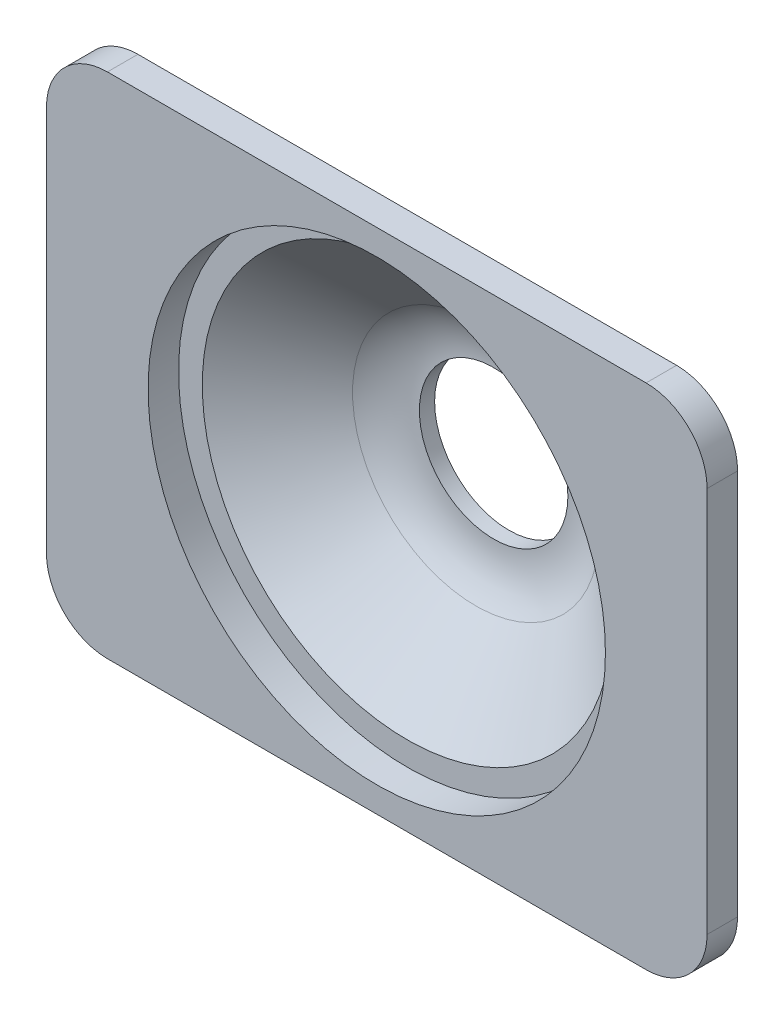
ISO-10303-21;
HEADER;
FILE_DESCRIPTION(('STEP AP214'),'2;1');
FILE_NAME('part.step','',(''),(''),'','','');
FILE_SCHEMA(('AUTOMOTIVE_DESIGN { 1 0 10303 214 1 1 1 1 }'));
ENDSEC;
DATA;
#1=APPLICATION_CONTEXT('core data for automotive mechanical design processes');
#2=APPLICATION_PROTOCOL_DEFINITION('international standard','automotive_design',2000,#1);
#3=PRODUCT_CONTEXT('',#1,'mechanical');
#4=PRODUCT('Part','Part','',(#3));
#5=PRODUCT_RELATED_PRODUCT_CATEGORY('part','',(#4));
#6=PRODUCT_DEFINITION_FORMATION('','',#4);
#7=PRODUCT_DEFINITION_CONTEXT('part definition',#1,'design');
#8=PRODUCT_DEFINITION('design','',#6,#7);
#9=PRODUCT_DEFINITION_SHAPE('','',#8);
#10=(LENGTH_UNIT() NAMED_UNIT(*) SI_UNIT(.MILLI.,.METRE.));
#11=(NAMED_UNIT(*) PLANE_ANGLE_UNIT() SI_UNIT($,.RADIAN.));
#12=(NAMED_UNIT(*) SI_UNIT($,.STERADIAN.) SOLID_ANGLE_UNIT());
#13=UNCERTAINTY_MEASURE_WITH_UNIT(LENGTH_MEASURE(1.E-05),#10,'distance_accuracy_value','');
#14=(GEOMETRIC_REPRESENTATION_CONTEXT(3) GLOBAL_UNCERTAINTY_ASSIGNED_CONTEXT((#13)) GLOBAL_UNIT_ASSIGNED_CONTEXT((#10,
#11,#12)) REPRESENTATION_CONTEXT('',''));
#15=CARTESIAN_POINT('',(0.,0.,0.));
#16=DIRECTION('',(0.,0.,1.));
#17=DIRECTION('',(1.,0.,0.));
#18=AXIS2_PLACEMENT_3D('',#15,#16,#17);
#19=CARTESIAN_POINT('',(-26.5,-19.,3.));
#20=DIRECTION('',(0.,0.,-1.));
#21=DIRECTION('',(-1.,0.,0.));
#22=AXIS2_PLACEMENT_3D('',#19,#20,#21);
#23=PLANE('',#22);
#24=CARTESIAN_POINT('',(-26.5,-19.,3.));
#25=DIRECTION('',(0.,0.,1.));
#26=DIRECTION('',(-1.,0.,0.));
#27=AXIS2_PLACEMENT_3D('',#24,#25,#26);
#28=CIRCLE('',#27,6.);
#29=CARTESIAN_POINT('',(-32.5,-19.,3.));
#30=VERTEX_POINT('',#29);
#31=CARTESIAN_POINT('',(-26.5,-25.,3.));
#32=VERTEX_POINT('',#31);
#33=EDGE_CURVE('E152',#30,#32,#28,.T.);
#34=ORIENTED_EDGE('',*,*,#33,.T.);
#35=DIRECTION('',(1.,0.,0.));
#36=VECTOR('',#35,1.);
#37=CARTESIAN_POINT('',(-26.5,-25.,3.));
#38=LINE('',#37,#36);
#39=CARTESIAN_POINT('',(26.5,-25.,3.));
#40=VERTEX_POINT('',#39);
#41=EDGE_CURVE('E100',#32,#40,#38,.T.);
#42=ORIENTED_EDGE('',*,*,#41,.T.);
#43=CARTESIAN_POINT('',(26.5,-19.,3.));
#44=DIRECTION('',(0.,0.,1.));
#45=DIRECTION('',(1.,0.,0.));
#46=AXIS2_PLACEMENT_3D('',#43,#44,#45);
#47=CIRCLE('',#46,6.);
#48=CARTESIAN_POINT('',(32.5,-19.,3.));
#49=VERTEX_POINT('',#48);
#50=EDGE_CURVE('E168',#40,#49,#47,.T.);
#51=ORIENTED_EDGE('',*,*,#50,.T.);
#52=DIRECTION('',(0.,1.,0.));
#53=VECTOR('',#52,1.);
#54=CARTESIAN_POINT('',(32.5,-19.,3.));
#55=LINE('',#54,#53);
#56=CARTESIAN_POINT('',(32.5,19.,3.));
#57=VERTEX_POINT('',#56);
#58=EDGE_CURVE('E178',#49,#57,#55,.T.);
#59=ORIENTED_EDGE('',*,*,#58,.T.);
#60=CARTESIAN_POINT('',(26.5,19.,3.));
#61=DIRECTION('',(0.,0.,1.));
#62=DIRECTION('',(-1.,0.,0.));
#63=AXIS2_PLACEMENT_3D('',#60,#61,#62);
#64=CIRCLE('',#63,6.);
#65=CARTESIAN_POINT('',(26.5,25.,3.));
#66=VERTEX_POINT('',#65);
#67=EDGE_CURVE('E117',#57,#66,#64,.T.);
#68=ORIENTED_EDGE('',*,*,#67,.T.);
#69=DIRECTION('',(-1.,0.,0.));
#70=VECTOR('',#69,1.);
#71=CARTESIAN_POINT('',(-26.5,25.,3.));
#72=LINE('',#71,#70);
#73=CARTESIAN_POINT('',(-26.5,25.,3.));
#74=VERTEX_POINT('',#73);
#75=EDGE_CURVE('E115',#66,#74,#72,.T.);
#76=ORIENTED_EDGE('',*,*,#75,.T.);
#77=CARTESIAN_POINT('',(-26.5,19.,3.));
#78=DIRECTION('',(0.,0.,1.));
#79=DIRECTION('',(-1.,0.,0.));
#80=AXIS2_PLACEMENT_3D('',#77,#78,#79);
#81=CIRCLE('',#80,6.);
#82=CARTESIAN_POINT('',(-32.5,19.,3.));
#83=VERTEX_POINT('',#82);
#84=EDGE_CURVE('E116',#74,#83,#81,.T.);
#85=ORIENTED_EDGE('',*,*,#84,.T.);
#86=DIRECTION('',(0.,-1.,0.));
#87=VECTOR('',#86,1.);
#88=CARTESIAN_POINT('',(-32.5,-19.,3.));
#89=LINE('',#88,#87);
#90=EDGE_CURVE('E57',#83,#30,#89,.T.);
#91=ORIENTED_EDGE('',*,*,#90,.T.);
#92=EDGE_LOOP('',(#34,#42,#51,#59,#68,#76,#85,#91));
#93=FACE_BOUND('',#92,.T.);
#94=CARTESIAN_POINT('',(0.,0.,3.));
#95=DIRECTION('',(0.,0.,1.));
#96=DIRECTION('',(1.,0.,0.));
#97=AXIS2_PLACEMENT_3D('',#94,#95,#96);
#98=CIRCLE('',#97,22.5);
#99=CARTESIAN_POINT('',(22.5,0.,3.));
#100=VERTEX_POINT('',#99);
#101=EDGE_CURVE('E137',#100,#100,#98,.T.);
#102=ORIENTED_EDGE('',*,*,#101,.F.);
#103=EDGE_LOOP('',(#102));
#104=FACE_BOUND('',#103,.T.);
#105=ADVANCED_FACE('F39',(#93,#104),#23,.F.);
#106=CARTESIAN_POINT('',(-26.5,-19.,0.));
#107=DIRECTION('',(0.,0.,-1.));
#108=DIRECTION('',(-1.,0.,0.));
#109=AXIS2_PLACEMENT_3D('',#106,#107,#108);
#110=PLANE('',#109);
#111=CARTESIAN_POINT('',(0.,0.,0.));
#112=DIRECTION('',(0.,0.,1.));
#113=DIRECTION('',(1.,0.,0.));
#114=AXIS2_PLACEMENT_3D('',#111,#112,#113);
#115=CIRCLE('',#114,24.6838214055972);
#116=CARTESIAN_POINT('',(24.6838214055972,0.,0.));
#117=VERTEX_POINT('',#116);
#118=EDGE_CURVE('E204',#117,#117,#115,.T.);
#119=ORIENTED_EDGE('',*,*,#118,.T.);
#120=EDGE_LOOP('',(#119));
#121=FACE_BOUND('',#120,.T.);
#122=CARTESIAN_POINT('',(-26.5,-19.,0.));
#123=DIRECTION('',(0.,0.,1.));
#124=DIRECTION('',(-1.,0.,0.));
#125=AXIS2_PLACEMENT_3D('',#122,#123,#124);
#126=CIRCLE('',#125,6.);
#127=CARTESIAN_POINT('',(-32.5,-19.,0.));
#128=VERTEX_POINT('',#127);
#129=CARTESIAN_POINT('',(-26.5,-25.,0.));
#130=VERTEX_POINT('',#129);
#131=EDGE_CURVE('E139',#128,#130,#126,.T.);
#132=ORIENTED_EDGE('',*,*,#131,.F.);
#133=DIRECTION('',(0.,-1.,0.));
#134=VECTOR('',#133,1.);
#135=CARTESIAN_POINT('',(-32.5,-19.,0.));
#136=LINE('',#135,#134);
#137=CARTESIAN_POINT('',(-32.5,19.,0.));
#138=VERTEX_POINT('',#137);
#139=EDGE_CURVE('E94',#138,#128,#136,.T.);
#140=ORIENTED_EDGE('',*,*,#139,.F.);
#141=CARTESIAN_POINT('',(-26.5,19.,0.));
#142=DIRECTION('',(0.,0.,1.));
#143=DIRECTION('',(-1.,0.,0.));
#144=AXIS2_PLACEMENT_3D('',#141,#142,#143);
#145=CIRCLE('',#144,6.);
#146=CARTESIAN_POINT('',(-26.5,25.,0.));
#147=VERTEX_POINT('',#146);
#148=EDGE_CURVE('E83',#147,#138,#145,.T.);
#149=ORIENTED_EDGE('',*,*,#148,.F.);
#150=DIRECTION('',(-1.,0.,0.));
#151=VECTOR('',#150,1.);
#152=CARTESIAN_POINT('',(-26.5,25.,0.));
#153=LINE('',#152,#151);
#154=CARTESIAN_POINT('',(26.5,25.,0.));
#155=VERTEX_POINT('',#154);
#156=EDGE_CURVE('E127',#155,#147,#153,.T.);
#157=ORIENTED_EDGE('',*,*,#156,.F.);
#158=CARTESIAN_POINT('',(26.5,19.,0.));
#159=DIRECTION('',(0.,0.,1.));
#160=DIRECTION('',(-1.,0.,0.));
#161=AXIS2_PLACEMENT_3D('',#158,#159,#160);
#162=CIRCLE('',#161,6.);
#163=CARTESIAN_POINT('',(32.5,19.,0.));
#164=VERTEX_POINT('',#163);
#165=EDGE_CURVE('E147',#164,#155,#162,.T.);
#166=ORIENTED_EDGE('',*,*,#165,.F.);
#167=DIRECTION('',(0.,1.,0.));
#168=VECTOR('',#167,1.);
#169=CARTESIAN_POINT('',(32.5,-19.,0.));
#170=LINE('',#169,#168);
#171=CARTESIAN_POINT('',(32.5,-19.,0.));
#172=VERTEX_POINT('',#171);
#173=EDGE_CURVE('E144',#172,#164,#170,.T.);
#174=ORIENTED_EDGE('',*,*,#173,.F.);
#175=CARTESIAN_POINT('',(26.5,-19.,0.));
#176=DIRECTION('',(0.,0.,1.));
#177=DIRECTION('',(1.,0.,0.));
#178=AXIS2_PLACEMENT_3D('',#175,#176,#177);
#179=CIRCLE('',#178,6.);
#180=CARTESIAN_POINT('',(26.5,-25.,0.));
#181=VERTEX_POINT('',#180);
#182=EDGE_CURVE('E145',#181,#172,#179,.T.);
#183=ORIENTED_EDGE('',*,*,#182,.F.);
#184=DIRECTION('',(1.,0.,0.));
#185=VECTOR('',#184,1.);
#186=CARTESIAN_POINT('',(-26.5,-25.,0.));
#187=LINE('',#186,#185);
#188=EDGE_CURVE('E138',#130,#181,#187,.T.);
#189=ORIENTED_EDGE('',*,*,#188,.F.);
#190=EDGE_LOOP('',(#132,#140,#149,#157,#166,#174,#183,#189));
#191=FACE_BOUND('',#190,.T.);
#192=ADVANCED_FACE('F167',(#121,#191),#110,.T.);
#193=CARTESIAN_POINT('',(-26.5,-19.,3.));
#194=DIRECTION('',(0.,0.,-1.));
#195=DIRECTION('',(-1.,0.,0.));
#196=AXIS2_PLACEMENT_3D('',#193,#194,#195);
#197=CYLINDRICAL_SURFACE('',#196,6.);
#198=ORIENTED_EDGE('',*,*,#131,.T.);
#199=DIRECTION('',(0.,0.,-1.));
#200=VECTOR('',#199,1.);
#201=CARTESIAN_POINT('',(-26.5,-25.,3.));
#202=LINE('',#201,#200);
#203=EDGE_CURVE('E11',#32,#130,#202,.T.);
#204=ORIENTED_EDGE('',*,*,#203,.F.);
#205=ORIENTED_EDGE('',*,*,#33,.F.);
#206=DIRECTION('',(0.,0.,-1.));
#207=VECTOR('',#206,1.);
#208=CARTESIAN_POINT('',(-32.5,-19.,3.));
#209=LINE('',#208,#207);
#210=EDGE_CURVE('E134',#30,#128,#209,.T.);
#211=ORIENTED_EDGE('',*,*,#210,.T.);
#212=EDGE_LOOP('',(#198,#204,#205,#211));
#213=FACE_BOUND('',#212,.T.);
#214=ADVANCED_FACE('F41',(#213),#197,.T.);
#215=CARTESIAN_POINT('',(-26.5,-25.,3.));
#216=DIRECTION('',(0.,1.,0.));
#217=DIRECTION('',(0.,0.,1.));
#218=AXIS2_PLACEMENT_3D('',#215,#216,#217);
#219=PLANE('',#218);
#220=ORIENTED_EDGE('',*,*,#188,.T.);
#221=DIRECTION('',(0.,0.,-1.));
#222=VECTOR('',#221,1.);
#223=CARTESIAN_POINT('',(26.5,-25.,3.));
#224=LINE('',#223,#222);
#225=EDGE_CURVE('E48',#40,#181,#224,.T.);
#226=ORIENTED_EDGE('',*,*,#225,.F.);
#227=ORIENTED_EDGE('',*,*,#41,.F.);
#228=ORIENTED_EDGE('',*,*,#203,.T.);
#229=EDGE_LOOP('',(#220,#226,#227,#228));
#230=FACE_BOUND('',#229,.T.);
#231=ADVANCED_FACE('F251',(#230),#219,.F.);
#232=CARTESIAN_POINT('',(26.5,-19.,3.));
#233=DIRECTION('',(0.,0.,-1.));
#234=DIRECTION('',(-1.,0.,0.));
#235=AXIS2_PLACEMENT_3D('',#232,#233,#234);
#236=CYLINDRICAL_SURFACE('',#235,6.);
#237=ORIENTED_EDGE('',*,*,#182,.T.);
#238=DIRECTION('',(0.,0.,-1.));
#239=VECTOR('',#238,1.);
#240=CARTESIAN_POINT('',(32.5,-19.,3.));
#241=LINE('',#240,#239);
#242=EDGE_CURVE('E160',#49,#172,#241,.T.);
#243=ORIENTED_EDGE('',*,*,#242,.F.);
#244=ORIENTED_EDGE('',*,*,#50,.F.);
#245=ORIENTED_EDGE('',*,*,#225,.T.);
#246=EDGE_LOOP('',(#237,#243,#244,#245));
#247=FACE_BOUND('',#246,.T.);
#248=ADVANCED_FACE('F165',(#247),#236,.T.);
#249=CARTESIAN_POINT('',(32.5,-19.,3.));
#250=DIRECTION('',(-1.,0.,0.));
#251=DIRECTION('',(0.,0.,1.));
#252=AXIS2_PLACEMENT_3D('',#249,#250,#251);
#253=PLANE('',#252);
#254=ORIENTED_EDGE('',*,*,#173,.T.);
#255=DIRECTION('',(0.,0.,-1.));
#256=VECTOR('',#255,1.);
#257=CARTESIAN_POINT('',(32.5,19.,3.));
#258=LINE('',#257,#256);
#259=EDGE_CURVE('E153',#57,#164,#258,.T.);
#260=ORIENTED_EDGE('',*,*,#259,.F.);
#261=ORIENTED_EDGE('',*,*,#58,.F.);
#262=ORIENTED_EDGE('',*,*,#242,.T.);
#263=EDGE_LOOP('',(#254,#260,#261,#262));
#264=FACE_BOUND('',#263,.T.);
#265=ADVANCED_FACE('F172',(#264),#253,.F.);
#266=CARTESIAN_POINT('',(26.5,19.,3.));
#267=DIRECTION('',(0.,0.,-1.));
#268=DIRECTION('',(-1.,0.,0.));
#269=AXIS2_PLACEMENT_3D('',#266,#267,#268);
#270=CYLINDRICAL_SURFACE('',#269,6.);
#271=ORIENTED_EDGE('',*,*,#165,.T.);
#272=DIRECTION('',(0.,0.,-1.));
#273=VECTOR('',#272,1.);
#274=CARTESIAN_POINT('',(26.5,25.,3.));
#275=LINE('',#274,#273);
#276=EDGE_CURVE('E130',#66,#155,#275,.T.);
#277=ORIENTED_EDGE('',*,*,#276,.F.);
#278=ORIENTED_EDGE('',*,*,#67,.F.);
#279=ORIENTED_EDGE('',*,*,#259,.T.);
#280=EDGE_LOOP('',(#271,#277,#278,#279));
#281=FACE_BOUND('',#280,.T.);
#282=ADVANCED_FACE('F180',(#281),#270,.T.);
#283=CARTESIAN_POINT('',(-26.5,25.,3.));
#284=DIRECTION('',(0.,-1.,0.));
#285=DIRECTION('',(0.,0.,-1.));
#286=AXIS2_PLACEMENT_3D('',#283,#284,#285);
#287=PLANE('',#286);
#288=ORIENTED_EDGE('',*,*,#156,.T.);
#289=DIRECTION('',(0.,0.,-1.));
#290=VECTOR('',#289,1.);
#291=CARTESIAN_POINT('',(-26.5,25.,3.));
#292=LINE('',#291,#290);
#293=EDGE_CURVE('E124',#74,#147,#292,.T.);
#294=ORIENTED_EDGE('',*,*,#293,.F.);
#295=ORIENTED_EDGE('',*,*,#75,.F.);
#296=ORIENTED_EDGE('',*,*,#276,.T.);
#297=EDGE_LOOP('',(#288,#294,#295,#296));
#298=FACE_BOUND('',#297,.T.);
#299=ADVANCED_FACE('F121',(#298),#287,.F.);
#300=CARTESIAN_POINT('',(-26.5,19.,3.));
#301=DIRECTION('',(0.,0.,-1.));
#302=DIRECTION('',(-1.,0.,0.));
#303=AXIS2_PLACEMENT_3D('',#300,#301,#302);
#304=CYLINDRICAL_SURFACE('',#303,6.);
#305=ORIENTED_EDGE('',*,*,#148,.T.);
#306=DIRECTION('',(0.,0.,-1.));
#307=VECTOR('',#306,1.);
#308=CARTESIAN_POINT('',(-32.5,19.,3.));
#309=LINE('',#308,#307);
#310=EDGE_CURVE('E129',#83,#138,#309,.T.);
#311=ORIENTED_EDGE('',*,*,#310,.F.);
#312=ORIENTED_EDGE('',*,*,#84,.F.);
#313=ORIENTED_EDGE('',*,*,#293,.T.);
#314=EDGE_LOOP('',(#305,#311,#312,#313));
#315=FACE_BOUND('',#314,.T.);
#316=ADVANCED_FACE('F128',(#315),#304,.T.);
#317=CARTESIAN_POINT('',(-32.5,-19.,3.));
#318=DIRECTION('',(1.,0.,0.));
#319=DIRECTION('',(0.,0.,-1.));
#320=AXIS2_PLACEMENT_3D('',#317,#318,#319);
#321=PLANE('',#320);
#322=ORIENTED_EDGE('',*,*,#139,.T.);
#323=ORIENTED_EDGE('',*,*,#210,.F.);
#324=ORIENTED_EDGE('',*,*,#90,.F.);
#325=ORIENTED_EDGE('',*,*,#310,.T.);
#326=EDGE_LOOP('',(#322,#323,#324,#325));
#327=FACE_BOUND('',#326,.T.);
#328=ADVANCED_FACE('F245',(#327),#321,.F.);
#329=CARTESIAN_POINT('',(0.,0.,3.));
#330=DIRECTION('',(0.,0.,-1.));
#331=DIRECTION('',(-1.,0.,0.));
#332=AXIS2_PLACEMENT_3D('',#329,#330,#331);
#333=CYLINDRICAL_SURFACE('',#332,22.5);
#334=ORIENTED_EDGE('',*,*,#101,.T.);
#335=EDGE_LOOP('',(#334));
#336=FACE_BOUND('',#335,.T.);
#337=CARTESIAN_POINT('',(0.,0.,0.));
#338=DIRECTION('',(0.,0.,1.));
#339=DIRECTION('',(1.,0.,0.));
#340=AXIS2_PLACEMENT_3D('',#337,#338,#339);
#341=CIRCLE('',#340,22.5);
#342=CARTESIAN_POINT('',(22.5,0.,0.));
#343=VERTEX_POINT('',#342);
#344=EDGE_CURVE('E183',#343,#343,#341,.T.);
#345=ORIENTED_EDGE('',*,*,#344,.F.);
#346=EDGE_LOOP('',(#345));
#347=FACE_BOUND('',#346,.T.);
#348=ADVANCED_FACE('F239',(#336,#347),#333,.F.);
#349=CARTESIAN_POINT('',(0.,0.,-1.));
#350=DIRECTION('',(0.,0.,1.));
#351=DIRECTION('',(1.,0.,0.));
#352=AXIS2_PLACEMENT_3D('',#349,#350,#351);
#353=DEGENERATE_TOROIDAL_SURFACE('',#352,7.30673196566218,7.5,.T.);
#354=CARTESIAN_POINT('',(0.,0.,-6.74533332339231));
#355=DIRECTION('',(0.,0.,1.));
#356=DIRECTION('',(1.,0.,0.));
#357=AXIS2_PLACEMENT_3D('',#354,#355,#356);
#358=CIRCLE('',#357,12.1276390383113);
#359=CARTESIAN_POINT('',(12.1276390383113,0.,-6.74533332339231));
#360=VERTEX_POINT('',#359);
#361=EDGE_CURVE('E195',#360,#360,#358,.T.);
#362=ORIENTED_EDGE('',*,*,#361,.T.);
#363=EDGE_LOOP('',(#362));
#364=FACE_BOUND('',#363,.T.);
#365=CARTESIAN_POINT('',(0.,0.,-8.5));
#366=DIRECTION('',(0.,0.,1.));
#367=DIRECTION('',(1.,0.,0.));
#368=AXIS2_PLACEMENT_3D('',#365,#366,#367);
#369=CIRCLE('',#368,7.30673196566218);
#370=CARTESIAN_POINT('',(7.30673196566218,0.,-8.5));
#371=VERTEX_POINT('',#370);
#372=EDGE_CURVE('E203',#371,#371,#369,.T.);
#373=ORIENTED_EDGE('',*,*,#372,.F.);
#374=EDGE_LOOP('',(#373));
#375=FACE_BOUND('',#374,.T.);
#376=ADVANCED_FACE('F320',(#364,#375),#353,.F.);
#377=CARTESIAN_POINT('',(0.,0.,-6.74533332339231));
#378=DIRECTION('',(0.,0.,1.));
#379=DIRECTION('',(1.,0.,0.));
#380=AXIS2_PLACEMENT_3D('',#377,#378,#379);
#381=CONICAL_SURFACE('',#380,12.1276390383113,0.872664625997159);
#382=CARTESIAN_POINT('',(0.,0.,0.));
#383=DIRECTION('',(0.,0.,1.));
#384=DIRECTION('',(1.,0.,0.));
#385=AXIS2_PLACEMENT_3D('',#382,#383,#384);
#386=CIRCLE('',#385,20.1664142597094);
#387=CARTESIAN_POINT('',(20.1664142597094,0.,0.));
#388=VERTEX_POINT('',#387);
#389=EDGE_CURVE('E190',#388,#388,#386,.T.);
#390=ORIENTED_EDGE('',*,*,#389,.T.);
#391=EDGE_LOOP('',(#390));
#392=FACE_BOUND('',#391,.T.);
#393=ORIENTED_EDGE('',*,*,#361,.F.);
#394=EDGE_LOOP('',(#393));
#395=FACE_BOUND('',#394,.T.);
#396=ADVANCED_FACE('F228',(#392,#395),#381,.F.);
#397=CARTESIAN_POINT('',(24.6838214055972,0.,0.));
#398=DIRECTION('',(0.,0.,-1.));
#399=DIRECTION('',(-1.,0.,0.));
#400=AXIS2_PLACEMENT_3D('',#397,#398,#399);
#401=PLANE('',#400);
#402=ORIENTED_EDGE('',*,*,#389,.F.);
#403=EDGE_LOOP('',(#402));
#404=FACE_BOUND('',#403,.T.);
#405=ORIENTED_EDGE('',*,*,#344,.T.);
#406=EDGE_LOOP('',(#405));
#407=FACE_BOUND('',#406,.T.);
#408=ADVANCED_FACE('F217',(#404,#407),#401,.F.);
#409=CARTESIAN_POINT('',(0.,0.,-1.));
#410=DIRECTION('',(0.,0.,1.));
#411=DIRECTION('',(1.,0.,0.));
#412=AXIS2_PLACEMENT_3D('',#409,#410,#411);
#413=DEGENERATE_TOROIDAL_SURFACE('',#412,7.30673196566218,9.,.T.);
#414=CARTESIAN_POINT('',(0.,0.,-7.89439998807077));
#415=DIRECTION('',(0.,0.,1.));
#416=DIRECTION('',(1.,0.,0.));
#417=AXIS2_PLACEMENT_3D('',#414,#415,#416);
#418=CIRCLE('',#417,13.0918204528411);
#419=CARTESIAN_POINT('',(13.0918204528411,0.,-7.89439998807077));
#420=VERTEX_POINT('',#419);
#421=EDGE_CURVE('E193',#420,#420,#418,.T.);
#422=ORIENTED_EDGE('',*,*,#421,.F.);
#423=EDGE_LOOP('',(#422));
#424=FACE_BOUND('',#423,.T.);
#425=CARTESIAN_POINT('',(0.,0.,-10.));
#426=DIRECTION('',(0.,0.,-1.));
#427=DIRECTION('',(-1.,0.,0.));
#428=AXIS2_PLACEMENT_3D('',#425,#426,#427);
#429=CIRCLE('',#428,7.30673196566218);
#430=CARTESIAN_POINT('',(-7.30673196566218,0.,-10.));
#431=VERTEX_POINT('',#430);
#432=EDGE_CURVE('E210',#431,#431,#429,.T.);
#433=ORIENTED_EDGE('',*,*,#432,.F.);
#434=EDGE_LOOP('',(#433));
#435=FACE_BOUND('',#434,.T.);
#436=ADVANCED_FACE('F214',(#424,#435),#413,.T.);
#437=CARTESIAN_POINT('',(0.,0.,-7.89439998807077));
#438=DIRECTION('',(0.,0.,1.));
#439=DIRECTION('',(1.,0.,0.));
#440=AXIS2_PLACEMENT_3D('',#437,#438,#439);
#441=CONICAL_SURFACE('',#440,13.0918204528411,0.87266462599716);
#442=CARTESIAN_POINT('',(0.,0.,-1.40373334128616));
#443=DIRECTION('',(0.,0.,1.));
#444=DIRECTION('',(1.,0.,0.));
#445=AXIS2_PLACEMENT_3D('',#442,#443,#444);
#446=CIRCLE('',#445,20.827095747478);
#447=CARTESIAN_POINT('',(20.827095747478,0.,-1.40373334128616));
#448=VERTEX_POINT('',#447);
#449=EDGE_CURVE('E200',#448,#448,#446,.T.);
#450=ORIENTED_EDGE('',*,*,#449,.F.);
#451=EDGE_LOOP('',(#450));
#452=FACE_BOUND('',#451,.T.);
#453=ORIENTED_EDGE('',*,*,#421,.T.);
#454=EDGE_LOOP('',(#453));
#455=FACE_BOUND('',#454,.T.);
#456=ADVANCED_FACE('F213',(#452,#455),#441,.T.);
#457=CARTESIAN_POINT('',(0.,0.,-6.));
#458=DIRECTION('',(0.,0.,1.));
#459=DIRECTION('',(1.,0.,0.));
#460=AXIS2_PLACEMENT_3D('',#457,#458,#459);
#461=TOROIDAL_SURFACE('',#460,24.6838214055972,6.);
#462=ORIENTED_EDGE('',*,*,#118,.F.);
#463=EDGE_LOOP('',(#462));
#464=FACE_BOUND('',#463,.T.);
#465=ORIENTED_EDGE('',*,*,#449,.T.);
#466=EDGE_LOOP('',(#465));
#467=FACE_BOUND('',#466,.T.);
#468=ADVANCED_FACE('F225',(#464,#467),#461,.F.);
#469=CARTESIAN_POINT('',(0.,0.,-7.));
#470=DIRECTION('',(0.,0.,-1.));
#471=DIRECTION('',(-1.,0.,0.));
#472=AXIS2_PLACEMENT_3D('',#469,#470,#471);
#473=CYLINDRICAL_SURFACE('',#472,7.30673196566218);
#474=ORIENTED_EDGE('',*,*,#372,.T.);
#475=EDGE_LOOP('',(#474));
#476=FACE_BOUND('',#475,.T.);
#477=ORIENTED_EDGE('',*,*,#432,.T.);
#478=EDGE_LOOP('',(#477));
#479=FACE_BOUND('',#478,.T.);
#480=ADVANCED_FACE('F212',(#476,#479),#473,.F.);
#481=CLOSED_SHELL('',(#105,#192,#214,#231,#248,#265,#282,#299,#316,#328,#348,#376,#396,#408,
#436,#456,#468,#480));
#482=MANIFOLD_SOLID_BREP('B2',#481);
#483=ADVANCED_BREP_SHAPE_REPRESENTATION('',(#18,#482),#14);
#484=SHAPE_DEFINITION_REPRESENTATION(#9,#483);
ENDSEC;
END-ISO-10303-21;
